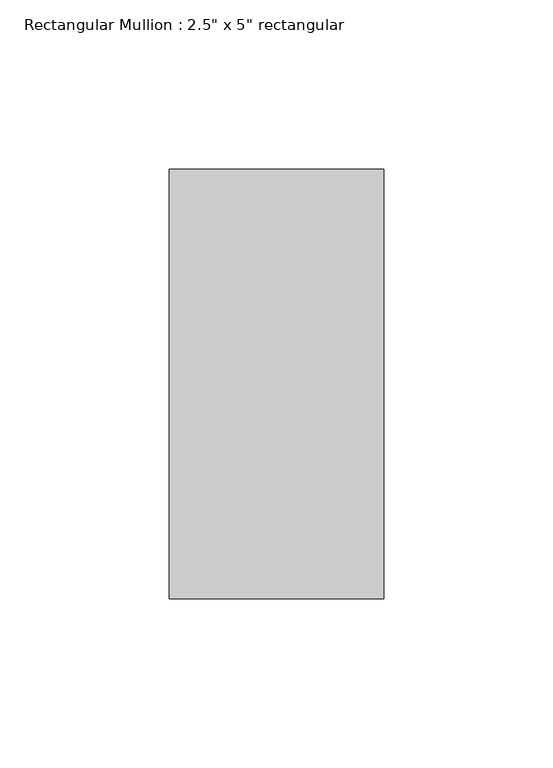
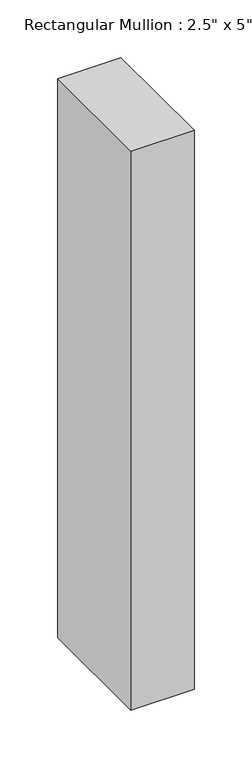
"""IFC4 building model written with IfcOpenShell, lengths in millimetres: member geometry."""

from ifc_helpers import new_model, si_unit, frame, origin, place, context, project, spatial, polyline, outline, extrude, source, transform, mapped, element, save


def member_c273ec95(model_context):
    return source(origin(), model_context, "Body", "SweptSolid", [
        extrude(outline(polyline([(31.75, 63.5), (31.75, -63.5), (-31.75, -63.5), (-31.75, 63.5), (31.75, 63.5)])), frame((0.0, 0.0, -592.655826), z_axis=(0.0, 0.0, 1.0), x_axis=(1.0, 0.0, 0.0)), (0.0, 0.0, 1.0), 592.655826),
    ])


if __name__ == "__main__":
    model = new_model("IFC4")
    model_context = context("Model", 3, world=origin())
    ifc_project = project(units=[si_unit("LENGTHUNIT", "METRE", prefix="MILLI")], contexts=[model_context])
    site = spatial("IfcSite", under=ifc_project)
    building = spatial("IfcBuilding", under=site)
    placement = place(None, origin())
    member_shape = member_c273ec95(model_context)
    element("IfcMember", 1, ObjectType="Rectangular Mullion : 2.5\" x 5\" rectangular", at=placement, inside=building, context=model_context, shape_type="MappedRepresentation", body=[
        mapped(member_shape, transform((0.0, 0.0, 0.0), x_axis=(1.0, 0.0, 0.0), y_axis=(0.0, 1.0, 0.0), z_axis=(0.0, 0.0, 1.0))),
    ])
    save(model, "model.ifc")

# Revit data of these elements
# Type "Rectangular Mullion : 2.5\" x 5\" rectangular"
#   built-in parameter 1007304 = 0.416667 (stored number, unit not read)
#   built-in parameter 1007301 = 0.104167 (stored number, unit not read)
#   built-in parameter 1007300 = 0.104167 (stored number, unit not read)
# Element 1 (IfcMember, "Rectangular Mullion : 2.5\" x 5\" rectangular")
#   Materials on its faces: "Aluminum"
# Materials
#   "Aluminum": class "Metal", colour RGB 247 247 247, transparency 0, Description = "Aluminum 6061", Cost = 0
